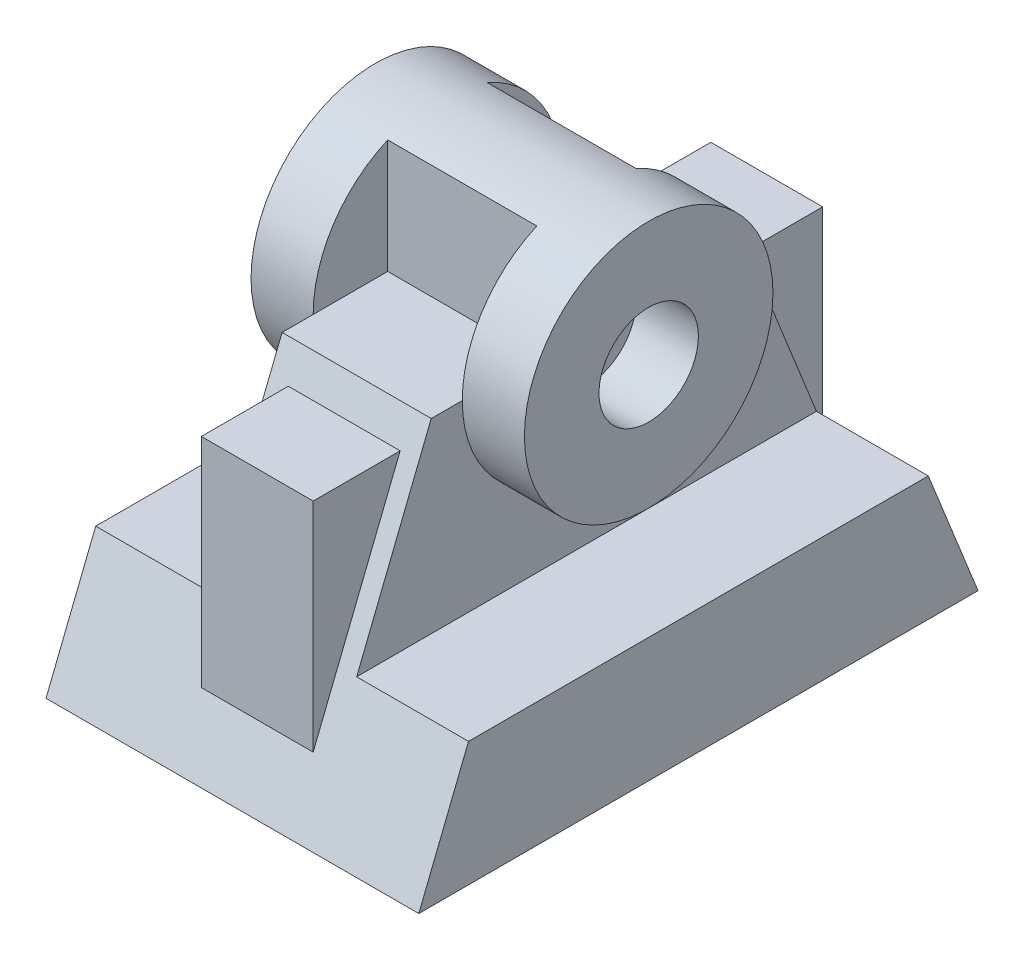
ISO-10303-21;
HEADER;
FILE_DESCRIPTION(('STEP AP214'),'2;1');
FILE_NAME('part.step','',(''),(''),'','','');
FILE_SCHEMA(('AUTOMOTIVE_DESIGN { 1 0 10303 214 1 1 1 1 }'));
ENDSEC;
DATA;
#1=APPLICATION_CONTEXT('core data for automotive mechanical design processes');
#2=APPLICATION_PROTOCOL_DEFINITION('international standard','automotive_design',2000,#1);
#3=PRODUCT_CONTEXT('',#1,'mechanical');
#4=PRODUCT('Part','Part','',(#3));
#5=PRODUCT_RELATED_PRODUCT_CATEGORY('part','',(#4));
#6=PRODUCT_DEFINITION_FORMATION('','',#4);
#7=PRODUCT_DEFINITION_CONTEXT('part definition',#1,'design');
#8=PRODUCT_DEFINITION('design','',#6,#7);
#9=PRODUCT_DEFINITION_SHAPE('','',#8);
#10=(LENGTH_UNIT() NAMED_UNIT(*) SI_UNIT(.MILLI.,.METRE.));
#11=(NAMED_UNIT(*) PLANE_ANGLE_UNIT() SI_UNIT($,.RADIAN.));
#12=(NAMED_UNIT(*) SI_UNIT($,.STERADIAN.) SOLID_ANGLE_UNIT());
#13=UNCERTAINTY_MEASURE_WITH_UNIT(LENGTH_MEASURE(1.E-05),#10,'distance_accuracy_value','');
#14=(GEOMETRIC_REPRESENTATION_CONTEXT(3) GLOBAL_UNCERTAINTY_ASSIGNED_CONTEXT((#13)) GLOBAL_UNIT_ASSIGNED_CONTEXT((#10,
#11,#12)) REPRESENTATION_CONTEXT('',''));
#15=CARTESIAN_POINT('',(0.,0.,0.));
#16=DIRECTION('',(0.,0.,1.));
#17=DIRECTION('',(1.,0.,0.));
#18=AXIS2_PLACEMENT_3D('',#15,#16,#17);
#19=CARTESIAN_POINT('',(22.,50.,0.));
#20=DIRECTION('',(-1.,0.,0.));
#21=DIRECTION('',(0.,0.,1.));
#22=AXIS2_PLACEMENT_3D('',#19,#20,#21);
#23=CYLINDRICAL_SURFACE('',#22,20.);
#24=CARTESIAN_POINT('',(-22.,50.,0.));
#25=DIRECTION('',(1.,0.,0.));
#26=DIRECTION('',(0.,0.,-1.));
#27=AXIS2_PLACEMENT_3D('',#24,#25,#26);
#28=CIRCLE('',#27,20.);
#29=CARTESIAN_POINT('',(-22.,50.,-20.));
#30=VERTEX_POINT('',#29);
#31=EDGE_CURVE('E228',#30,#30,#28,.T.);
#32=ORIENTED_EDGE('',*,*,#31,.T.);
#33=EDGE_LOOP('',(#32));
#34=FACE_BOUND('',#33,.T.);
#35=CARTESIAN_POINT('',(22.,50.,0.));
#36=DIRECTION('',(1.,0.,0.));
#37=DIRECTION('',(0.,0.,-1.));
#38=AXIS2_PLACEMENT_3D('',#35,#36,#37);
#39=CIRCLE('',#38,20.);
#40=CARTESIAN_POINT('',(22.,50.,-20.));
#41=VERTEX_POINT('',#40);
#42=EDGE_CURVE('E226',#41,#41,#39,.T.);
#43=ORIENTED_EDGE('',*,*,#42,.F.);
#44=EDGE_LOOP('',(#43));
#45=FACE_BOUND('',#44,.T.);
#46=CARTESIAN_POINT('',(12.,50.,0.));
#47=DIRECTION('',(-1.,0.,0.));
#48=DIRECTION('',(0.,0.,1.));
#49=AXIS2_PLACEMENT_3D('',#46,#47,#48);
#50=CIRCLE('',#49,20.);
#51=CARTESIAN_POINT('',(12.,68.3303027798234,-8.00000000000001));
#52=VERTEX_POINT('',#51);
#53=CARTESIAN_POINT('',(12.,50.,-20.));
#54=VERTEX_POINT('',#53);
#55=EDGE_CURVE('E199',#52,#54,#50,.T.);
#56=ORIENTED_EDGE('',*,*,#55,.F.);
#57=DIRECTION('',(1.,0.,0.));
#58=VECTOR('',#57,1.);
#59=CARTESIAN_POINT('',(-12.,68.3303027798234,-8.00000000000001));
#60=LINE('',#59,#58);
#61=CARTESIAN_POINT('',(-12.,68.3303027798234,-8.00000000000001));
#62=VERTEX_POINT('',#61);
#63=EDGE_CURVE('E183',#62,#52,#60,.T.);
#64=ORIENTED_EDGE('',*,*,#63,.F.);
#65=CARTESIAN_POINT('',(-12.,50.,0.));
#66=DIRECTION('',(-1.,0.,0.));
#67=DIRECTION('',(0.,0.,1.));
#68=AXIS2_PLACEMENT_3D('',#65,#66,#67);
#69=CIRCLE('',#68,20.);
#70=CARTESIAN_POINT('',(-12.,50.,-20.));
#71=VERTEX_POINT('',#70);
#72=EDGE_CURVE('E53',#62,#71,#69,.T.);
#73=ORIENTED_EDGE('',*,*,#72,.T.);
#74=CARTESIAN_POINT('',(-12.,50.,0.));
#75=DIRECTION('',(1.,0.,0.));
#76=DIRECTION('',(0.,0.,-1.));
#77=AXIS2_PLACEMENT_3D('',#74,#75,#76);
#78=CIRCLE('',#77,20.);
#79=CARTESIAN_POINT('',(-12.,50.,20.));
#80=VERTEX_POINT('',#79);
#81=EDGE_CURVE('E233',#71,#80,#78,.F.);
#82=ORIENTED_EDGE('',*,*,#81,.T.);
#83=CARTESIAN_POINT('',(-12.,50.,0.));
#84=DIRECTION('',(1.,0.,0.));
#85=DIRECTION('',(0.,0.,-1.));
#86=AXIS2_PLACEMENT_3D('',#83,#84,#85);
#87=CIRCLE('',#86,20.);
#88=CARTESIAN_POINT('',(-12.,68.3303027798234,8.00000000000001));
#89=VERTEX_POINT('',#88);
#90=EDGE_CURVE('E210',#89,#80,#87,.T.);
#91=ORIENTED_EDGE('',*,*,#90,.F.);
#92=DIRECTION('',(1.,0.,0.));
#93=VECTOR('',#92,1.);
#94=CARTESIAN_POINT('',(-12.,68.3303027798234,8.00000000000001));
#95=LINE('',#94,#93);
#96=CARTESIAN_POINT('',(12.,68.3303027798234,8.00000000000001));
#97=VERTEX_POINT('',#96);
#98=EDGE_CURVE('E222',#89,#97,#95,.T.);
#99=ORIENTED_EDGE('',*,*,#98,.T.);
#100=CARTESIAN_POINT('',(12.,50.,0.));
#101=DIRECTION('',(1.,0.,0.));
#102=DIRECTION('',(0.,0.,-1.));
#103=AXIS2_PLACEMENT_3D('',#100,#101,#102);
#104=CIRCLE('',#103,20.);
#105=CARTESIAN_POINT('',(12.,50.,20.));
#106=VERTEX_POINT('',#105);
#107=EDGE_CURVE('E195',#97,#106,#104,.T.);
#108=ORIENTED_EDGE('',*,*,#107,.T.);
#109=CARTESIAN_POINT('',(12.,50.,0.));
#110=DIRECTION('',(-1.,0.,0.));
#111=DIRECTION('',(0.,0.,1.));
#112=AXIS2_PLACEMENT_3D('',#109,#110,#111);
#113=CIRCLE('',#112,20.);
#114=EDGE_CURVE('E11',#106,#54,#113,.F.);
#115=ORIENTED_EDGE('',*,*,#114,.T.);
#116=EDGE_LOOP('',(#56,#64,#73,#82,#91,#99,#108,#115));
#117=FACE_BOUND('',#116,.T.);
#118=ADVANCED_FACE('F39',(#34,#45,#117),#23,.T.);
#119=CARTESIAN_POINT('',(30.,50.,25.));
#120=DIRECTION('',(0.,-1.,0.));
#121=DIRECTION('',(0.,0.,-1.));
#122=AXIS2_PLACEMENT_3D('',#119,#120,#121);
#123=PLANE('',#122);
#124=DIRECTION('',(0.,0.,-1.));
#125=VECTOR('',#124,1.);
#126=CARTESIAN_POINT('',(12.,50.,0.));
#127=LINE('',#126,#125);
#128=CARTESIAN_POINT('',(12.,50.,25.));
#129=VERTEX_POINT('',#128);
#130=EDGE_CURVE('E281',#129,#106,#127,.T.);
#131=ORIENTED_EDGE('',*,*,#130,.T.);
#132=DIRECTION('',(0.,0.,-1.));
#133=VECTOR('',#132,1.);
#134=CARTESIAN_POINT('',(12.,50.,8.00000000000001));
#135=LINE('',#134,#133);
#136=CARTESIAN_POINT('',(12.,50.,8.00000000000001));
#137=VERTEX_POINT('',#136);
#138=EDGE_CURVE('E218',#106,#137,#135,.T.);
#139=ORIENTED_EDGE('',*,*,#138,.T.);
#140=DIRECTION('',(1.,0.,0.));
#141=VECTOR('',#140,1.);
#142=CARTESIAN_POINT('',(-12.,50.,8.00000000000001));
#143=LINE('',#142,#141);
#144=CARTESIAN_POINT('',(-12.,50.,8.00000000000001));
#145=VERTEX_POINT('',#144);
#146=EDGE_CURVE('E216',#145,#137,#143,.T.);
#147=ORIENTED_EDGE('',*,*,#146,.F.);
#148=DIRECTION('',(0.,0.,-1.));
#149=VECTOR('',#148,1.);
#150=CARTESIAN_POINT('',(-12.,50.,8.00000000000001));
#151=LINE('',#150,#149);
#152=EDGE_CURVE('E208',#80,#145,#151,.T.);
#153=ORIENTED_EDGE('',*,*,#152,.F.);
#154=DIRECTION('',(0.,0.,1.));
#155=VECTOR('',#154,1.);
#156=CARTESIAN_POINT('',(-12.,50.,0.));
#157=LINE('',#156,#155);
#158=CARTESIAN_POINT('',(-12.,50.,25.));
#159=VERTEX_POINT('',#158);
#160=EDGE_CURVE('E300',#80,#159,#157,.T.);
#161=ORIENTED_EDGE('',*,*,#160,.T.);
#162=DIRECTION('',(-1.,0.,0.));
#163=VECTOR('',#162,1.);
#164=CARTESIAN_POINT('',(30.,50.,25.));
#165=LINE('',#164,#163);
#166=EDGE_CURVE('E335',#129,#159,#165,.T.);
#167=ORIENTED_EDGE('',*,*,#166,.F.);
#168=EDGE_LOOP('',(#131,#139,#147,#153,#161,#167));
#169=FACE_BOUND('',#168,.T.);
#170=ADVANCED_FACE('F374',(#169),#123,.F.);
#171=CARTESIAN_POINT('',(-12.,50.,-25.));
#172=VERTEX_POINT('',#171);
#173=EDGE_CURVE('E182',#172,#71,#157,.T.);
#174=ORIENTED_EDGE('',*,*,#173,.T.);
#175=DIRECTION('',(0.,0.,1.));
#176=VECTOR('',#175,1.);
#177=CARTESIAN_POINT('',(-12.,50.,-8.00000000000001));
#178=LINE('',#177,#176);
#179=CARTESIAN_POINT('',(-12.,50.,-8.00000000000001));
#180=VERTEX_POINT('',#179);
#181=EDGE_CURVE('E180',#71,#180,#178,.T.);
#182=ORIENTED_EDGE('',*,*,#181,.T.);
#183=DIRECTION('',(1.,0.,0.));
#184=VECTOR('',#183,1.);
#185=CARTESIAN_POINT('',(-12.,50.,-8.00000000000001));
#186=LINE('',#185,#184);
#187=CARTESIAN_POINT('',(12.,50.,-8.00000000000001));
#188=VERTEX_POINT('',#187);
#189=EDGE_CURVE('E179',#180,#188,#186,.T.);
#190=ORIENTED_EDGE('',*,*,#189,.T.);
#191=DIRECTION('',(0.,0.,1.));
#192=VECTOR('',#191,1.);
#193=CARTESIAN_POINT('',(12.,50.,-8.00000000000001));
#194=LINE('',#193,#192);
#195=EDGE_CURVE('E196',#54,#188,#194,.T.);
#196=ORIENTED_EDGE('',*,*,#195,.F.);
#197=CARTESIAN_POINT('',(12.,50.,-25.));
#198=VERTEX_POINT('',#197);
#199=EDGE_CURVE('E278',#54,#198,#127,.T.);
#200=ORIENTED_EDGE('',*,*,#199,.T.);
#201=DIRECTION('',(-1.,0.,0.));
#202=VECTOR('',#201,1.);
#203=CARTESIAN_POINT('',(30.,50.,-25.));
#204=LINE('',#203,#202);
#205=EDGE_CURVE('E334',#198,#172,#204,.T.);
#206=ORIENTED_EDGE('',*,*,#205,.T.);
#207=EDGE_LOOP('',(#174,#182,#190,#196,#200,#206));
#208=FACE_BOUND('',#207,.T.);
#209=ADVANCED_FACE('F177',(#208),#123,.F.);
#210=CARTESIAN_POINT('',(30.,0.,0.));
#211=DIRECTION('',(1.,0.,0.));
#212=DIRECTION('',(0.,0.,-1.));
#213=AXIS2_PLACEMENT_3D('',#210,#211,#212);
#214=PLANE('',#213);
#215=DIRECTION('',(0.,0.928476690885259,0.371390676354104));
#216=VECTOR('',#215,1.);
#217=CARTESIAN_POINT('',(30.,0.,-45.));
#218=LINE('',#217,#216);
#219=CARTESIAN_POINT('',(30.,0.,-45.));
#220=VERTEX_POINT('',#219);
#221=CARTESIAN_POINT('',(30.,20.,-37.));
#222=VERTEX_POINT('',#221);
#223=EDGE_CURVE('E312',#220,#222,#218,.T.);
#224=ORIENTED_EDGE('',*,*,#223,.T.);
#225=DIRECTION('',(0.,0.,1.));
#226=VECTOR('',#225,1.);
#227=CARTESIAN_POINT('',(30.,20.,0.));
#228=LINE('',#227,#226);
#229=CARTESIAN_POINT('',(30.,20.,37.));
#230=VERTEX_POINT('',#229);
#231=EDGE_CURVE('E271',#222,#230,#228,.T.);
#232=ORIENTED_EDGE('',*,*,#231,.T.);
#233=DIRECTION('',(0.,-0.928476690885259,0.371390676354104));
#234=VECTOR('',#233,1.);
#235=CARTESIAN_POINT('',(30.,0.,45.));
#236=LINE('',#235,#234);
#237=CARTESIAN_POINT('',(30.,0.,45.));
#238=VERTEX_POINT('',#237);
#239=EDGE_CURVE('E317',#230,#238,#236,.T.);
#240=ORIENTED_EDGE('',*,*,#239,.T.);
#241=DIRECTION('',(0.,0.,-1.));
#242=VECTOR('',#241,1.);
#243=CARTESIAN_POINT('',(30.,0.,45.));
#244=LINE('',#243,#242);
#245=EDGE_CURVE('E316',#238,#220,#244,.T.);
#246=ORIENTED_EDGE('',*,*,#245,.T.);
#247=EDGE_LOOP('',(#224,#232,#240,#246));
#248=FACE_BOUND('',#247,.T.);
#249=ADVANCED_FACE('F428',(#248),#214,.T.);
#250=CARTESIAN_POINT('',(30.,0.,-45.));
#251=DIRECTION('',(0.,-0.371390676354104,0.928476690885259));
#252=DIRECTION('',(0.,-0.928476690885259,-0.371390676354104));
#253=AXIS2_PLACEMENT_3D('',#250,#251,#252);
#254=PLANE('',#253);
#255=DIRECTION('',(-1.,0.,0.));
#256=VECTOR('',#255,1.);
#257=CARTESIAN_POINT('',(9.,9.99999999999999,-41.));
#258=LINE('',#257,#256);
#259=CARTESIAN_POINT('',(9.,10.,-41.));
#260=VERTEX_POINT('',#259);
#261=CARTESIAN_POINT('',(-9.,9.99999999999999,-41.));
#262=VERTEX_POINT('',#261);
#263=EDGE_CURVE('E258',#260,#262,#258,.T.);
#264=ORIENTED_EDGE('',*,*,#263,.F.);
#265=DIRECTION('',(0.,0.928476690885259,0.371390676354104));
#266=VECTOR('',#265,1.);
#267=CARTESIAN_POINT('',(9.,0.,-45.));
#268=LINE('',#267,#266);
#269=CARTESIAN_POINT('',(9.,45.,-27.));
#270=VERTEX_POINT('',#269);
#271=EDGE_CURVE('E267',#260,#270,#268,.T.);
#272=ORIENTED_EDGE('',*,*,#271,.T.);
#273=DIRECTION('',(1.,0.,0.));
#274=VECTOR('',#273,1.);
#275=CARTESIAN_POINT('',(30.,45.,-27.));
#276=LINE('',#275,#274);
#277=CARTESIAN_POINT('',(-9.,45.,-27.));
#278=VERTEX_POINT('',#277);
#279=EDGE_CURVE('E269',#278,#270,#276,.T.);
#280=ORIENTED_EDGE('',*,*,#279,.F.);
#281=DIRECTION('',(0.,0.928476690885259,0.371390676354104));
#282=VECTOR('',#281,1.);
#283=CARTESIAN_POINT('',(-9.,0.,-45.));
#284=LINE('',#283,#282);
#285=EDGE_CURVE('E264',#262,#278,#284,.T.);
#286=ORIENTED_EDGE('',*,*,#285,.F.);
#287=EDGE_LOOP('',(#264,#272,#280,#286));
#288=FACE_BOUND('',#287,.T.);
#289=DIRECTION('',(0.,-0.928476690885259,-0.371390676354104));
#290=VECTOR('',#289,1.);
#291=CARTESIAN_POINT('',(12.,15.5172413793103,-38.7931034482759));
#292=LINE('',#291,#290);
#293=CARTESIAN_POINT('',(12.,20.,-37.));
#294=VERTEX_POINT('',#293);
#295=EDGE_CURVE('E283',#198,#294,#292,.T.);
#296=ORIENTED_EDGE('',*,*,#295,.T.);
#297=DIRECTION('',(1.,0.,0.));
#298=VECTOR('',#297,1.);
#299=CARTESIAN_POINT('',(12.,20.,-37.));
#300=LINE('',#299,#298);
#301=EDGE_CURVE('E290',#294,#222,#300,.T.);
#302=ORIENTED_EDGE('',*,*,#301,.T.);
#303=ORIENTED_EDGE('',*,*,#223,.F.);
#304=DIRECTION('',(-1.,0.,0.));
#305=VECTOR('',#304,1.);
#306=CARTESIAN_POINT('',(30.,0.,-45.));
#307=LINE('',#306,#305);
#308=CARTESIAN_POINT('',(-30.,0.,-45.));
#309=VERTEX_POINT('',#308);
#310=EDGE_CURVE('E322',#220,#309,#307,.T.);
#311=ORIENTED_EDGE('',*,*,#310,.T.);
#312=DIRECTION('',(0.,0.928476690885259,0.371390676354104));
#313=VECTOR('',#312,1.);
#314=CARTESIAN_POINT('',(-30.,0.,-45.));
#315=LINE('',#314,#313);
#316=CARTESIAN_POINT('',(-30.,20.,-37.));
#317=VERTEX_POINT('',#316);
#318=EDGE_CURVE('E315',#309,#317,#315,.T.);
#319=ORIENTED_EDGE('',*,*,#318,.T.);
#320=DIRECTION('',(-1.,0.,0.));
#321=VECTOR('',#320,1.);
#322=CARTESIAN_POINT('',(-12.,20.,-37.));
#323=LINE('',#322,#321);
#324=CARTESIAN_POINT('',(-12.,20.,-37.));
#325=VERTEX_POINT('',#324);
#326=EDGE_CURVE('E304',#325,#317,#323,.T.);
#327=ORIENTED_EDGE('',*,*,#326,.F.);
#328=DIRECTION('',(0.,0.928476690885259,0.371390676354104));
#329=VECTOR('',#328,1.);
#330=CARTESIAN_POINT('',(-12.,15.5172413793103,-38.7931034482759));
#331=LINE('',#330,#329);
#332=EDGE_CURVE('E305',#325,#172,#331,.T.);
#333=ORIENTED_EDGE('',*,*,#332,.T.);
#334=ORIENTED_EDGE('',*,*,#205,.F.);
#335=EDGE_LOOP('',(#296,#302,#303,#311,#319,#327,#333,#334));
#336=FACE_BOUND('',#335,.T.);
#337=ADVANCED_FACE('F41',(#288,#336),#254,.F.);
#338=CARTESIAN_POINT('',(30.,0.,45.));
#339=DIRECTION('',(0.,-0.371390676354104,-0.928476690885259));
#340=DIRECTION('',(0.,0.928476690885259,-0.371390676354104));
#341=AXIS2_PLACEMENT_3D('',#338,#339,#340);
#342=PLANE('',#341);
#343=DIRECTION('',(-1.,0.,0.));
#344=VECTOR('',#343,1.);
#345=CARTESIAN_POINT('',(30.,45.,27.));
#346=LINE('',#345,#344);
#347=CARTESIAN_POINT('',(9.,45.,27.));
#348=VERTEX_POINT('',#347);
#349=CARTESIAN_POINT('',(-9.,45.,27.));
#350=VERTEX_POINT('',#349);
#351=EDGE_CURVE('E338',#348,#350,#346,.T.);
#352=ORIENTED_EDGE('',*,*,#351,.F.);
#353=DIRECTION('',(0.,-0.928476690885259,0.371390676354104));
#354=VECTOR('',#353,1.);
#355=CARTESIAN_POINT('',(9.,0.,45.));
#356=LINE('',#355,#354);
#357=CARTESIAN_POINT('',(9.,9.99999999999999,41.));
#358=VERTEX_POINT('',#357);
#359=EDGE_CURVE('E50',#348,#358,#356,.T.);
#360=ORIENTED_EDGE('',*,*,#359,.T.);
#361=DIRECTION('',(-1.,0.,0.));
#362=VECTOR('',#361,1.);
#363=CARTESIAN_POINT('',(9.,9.99999999999999,41.));
#364=LINE('',#363,#362);
#365=CARTESIAN_POINT('',(-9.,9.99999999999999,41.));
#366=VERTEX_POINT('',#365);
#367=EDGE_CURVE('E262',#358,#366,#364,.T.);
#368=ORIENTED_EDGE('',*,*,#367,.T.);
#369=DIRECTION('',(0.,-0.928476690885259,0.371390676354104));
#370=VECTOR('',#369,1.);
#371=CARTESIAN_POINT('',(-9.,0.,45.));
#372=LINE('',#371,#370);
#373=EDGE_CURVE('E340',#350,#366,#372,.T.);
#374=ORIENTED_EDGE('',*,*,#373,.F.);
#375=EDGE_LOOP('',(#352,#360,#368,#374));
#376=FACE_BOUND('',#375,.T.);
#377=DIRECTION('',(1.,0.,0.));
#378=VECTOR('',#377,1.);
#379=CARTESIAN_POINT('',(12.,20.,37.));
#380=LINE('',#379,#378);
#381=CARTESIAN_POINT('',(12.,20.,37.));
#382=VERTEX_POINT('',#381);
#383=EDGE_CURVE('E292',#382,#230,#380,.T.);
#384=ORIENTED_EDGE('',*,*,#383,.F.);
#385=DIRECTION('',(0.,0.928476690885259,-0.371390676354104));
#386=VECTOR('',#385,1.);
#387=CARTESIAN_POINT('',(12.,15.5172413793104,38.7931034482759));
#388=LINE('',#387,#386);
#389=EDGE_CURVE('E280',#382,#129,#388,.T.);
#390=ORIENTED_EDGE('',*,*,#389,.T.);
#391=ORIENTED_EDGE('',*,*,#166,.T.);
#392=DIRECTION('',(0.,-0.928476690885259,0.371390676354104));
#393=VECTOR('',#392,1.);
#394=CARTESIAN_POINT('',(-12.,15.5172413793104,38.7931034482759));
#395=LINE('',#394,#393);
#396=CARTESIAN_POINT('',(-12.,20.,37.));
#397=VERTEX_POINT('',#396);
#398=EDGE_CURVE('E298',#159,#397,#395,.T.);
#399=ORIENTED_EDGE('',*,*,#398,.T.);
#400=DIRECTION('',(-1.,0.,0.));
#401=VECTOR('',#400,1.);
#402=CARTESIAN_POINT('',(-12.,20.,37.));
#403=LINE('',#402,#401);
#404=CARTESIAN_POINT('',(-30.,20.,37.));
#405=VERTEX_POINT('',#404);
#406=EDGE_CURVE('E307',#397,#405,#403,.T.);
#407=ORIENTED_EDGE('',*,*,#406,.T.);
#408=DIRECTION('',(0.,-0.928476690885259,0.371390676354104));
#409=VECTOR('',#408,1.);
#410=CARTESIAN_POINT('',(-30.,0.,45.));
#411=LINE('',#410,#409);
#412=CARTESIAN_POINT('',(-30.,0.,45.));
#413=VERTEX_POINT('',#412);
#414=EDGE_CURVE('E321',#405,#413,#411,.T.);
#415=ORIENTED_EDGE('',*,*,#414,.T.);
#416=DIRECTION('',(-1.,0.,0.));
#417=VECTOR('',#416,1.);
#418=CARTESIAN_POINT('',(30.,0.,45.));
#419=LINE('',#418,#417);
#420=EDGE_CURVE('E328',#238,#413,#419,.T.);
#421=ORIENTED_EDGE('',*,*,#420,.F.);
#422=ORIENTED_EDGE('',*,*,#239,.F.);
#423=EDGE_LOOP('',(#384,#390,#391,#399,#407,#415,#421,#422));
#424=FACE_BOUND('',#423,.T.);
#425=ADVANCED_FACE('F341',(#376,#424),#342,.F.);
#426=CARTESIAN_POINT('',(30.,0.,45.));
#427=DIRECTION('',(0.,1.,0.));
#428=DIRECTION('',(0.,0.,1.));
#429=AXIS2_PLACEMENT_3D('',#426,#427,#428);
#430=PLANE('',#429);
#431=DIRECTION('',(0.,0.,-1.));
#432=VECTOR('',#431,1.);
#433=CARTESIAN_POINT('',(-30.,0.,45.));
#434=LINE('',#433,#432);
#435=EDGE_CURVE('E320',#413,#309,#434,.T.);
#436=ORIENTED_EDGE('',*,*,#435,.T.);
#437=ORIENTED_EDGE('',*,*,#310,.F.);
#438=ORIENTED_EDGE('',*,*,#245,.F.);
#439=ORIENTED_EDGE('',*,*,#420,.T.);
#440=EDGE_LOOP('',(#436,#437,#438,#439));
#441=FACE_BOUND('',#440,.T.);
#442=ADVANCED_FACE('F435',(#441),#430,.F.);
#443=CARTESIAN_POINT('',(-30.,0.,0.));
#444=DIRECTION('',(1.,0.,0.));
#445=DIRECTION('',(0.,0.,-1.));
#446=AXIS2_PLACEMENT_3D('',#443,#444,#445);
#447=PLANE('',#446);
#448=ORIENTED_EDGE('',*,*,#414,.F.);
#449=DIRECTION('',(0.,0.,-1.));
#450=VECTOR('',#449,1.);
#451=CARTESIAN_POINT('',(-30.,20.,0.));
#452=LINE('',#451,#450);
#453=EDGE_CURVE('E295',#405,#317,#452,.T.);
#454=ORIENTED_EDGE('',*,*,#453,.T.);
#455=ORIENTED_EDGE('',*,*,#318,.F.);
#456=ORIENTED_EDGE('',*,*,#435,.F.);
#457=EDGE_LOOP('',(#448,#454,#455,#456));
#458=FACE_BOUND('',#457,.T.);
#459=ADVANCED_FACE('F425',(#458),#447,.F.);
#460=CARTESIAN_POINT('',(-12.,20.,0.));
#461=DIRECTION('',(0.,1.,0.));
#462=DIRECTION('',(0.,0.,1.));
#463=AXIS2_PLACEMENT_3D('',#460,#461,#462);
#464=PLANE('',#463);
#465=ORIENTED_EDGE('',*,*,#453,.F.);
#466=ORIENTED_EDGE('',*,*,#406,.F.);
#467=DIRECTION('',(0.,0.,-1.));
#468=VECTOR('',#467,1.);
#469=CARTESIAN_POINT('',(-12.,20.,0.));
#470=LINE('',#469,#468);
#471=EDGE_CURVE('E297',#397,#325,#470,.T.);
#472=ORIENTED_EDGE('',*,*,#471,.T.);
#473=ORIENTED_EDGE('',*,*,#326,.T.);
#474=EDGE_LOOP('',(#465,#466,#472,#473));
#475=FACE_BOUND('',#474,.T.);
#476=ADVANCED_FACE('F419',(#475),#464,.T.);
#477=CARTESIAN_POINT('',(-12.,0.,0.));
#478=DIRECTION('',(1.,0.,0.));
#479=DIRECTION('',(0.,0.,-1.));
#480=AXIS2_PLACEMENT_3D('',#477,#478,#479);
#481=PLANE('',#480);
#482=ORIENTED_EDGE('',*,*,#81,.F.);
#483=ORIENTED_EDGE('',*,*,#173,.F.);
#484=ORIENTED_EDGE('',*,*,#332,.F.);
#485=ORIENTED_EDGE('',*,*,#471,.F.);
#486=ORIENTED_EDGE('',*,*,#398,.F.);
#487=ORIENTED_EDGE('',*,*,#160,.F.);
#488=EDGE_LOOP('',(#482,#483,#484,#485,#486,#487));
#489=FACE_BOUND('',#488,.T.);
#490=ADVANCED_FACE('F413',(#489),#481,.F.);
#491=CARTESIAN_POINT('',(12.,20.,0.));
#492=DIRECTION('',(0.,1.,0.));
#493=DIRECTION('',(0.,0.,1.));
#494=AXIS2_PLACEMENT_3D('',#491,#492,#493);
#495=PLANE('',#494);
#496=ORIENTED_EDGE('',*,*,#231,.F.);
#497=ORIENTED_EDGE('',*,*,#301,.F.);
#498=DIRECTION('',(0.,0.,1.));
#499=VECTOR('',#498,1.);
#500=CARTESIAN_POINT('',(12.,20.,0.));
#501=LINE('',#500,#499);
#502=EDGE_CURVE('E274',#294,#382,#501,.T.);
#503=ORIENTED_EDGE('',*,*,#502,.T.);
#504=ORIENTED_EDGE('',*,*,#383,.T.);
#505=EDGE_LOOP('',(#496,#497,#503,#504));
#506=FACE_BOUND('',#505,.T.);
#507=ADVANCED_FACE('F407',(#506),#495,.T.);
#508=CARTESIAN_POINT('',(12.,0.,0.));
#509=DIRECTION('',(-1.,0.,0.));
#510=DIRECTION('',(0.,0.,1.));
#511=AXIS2_PLACEMENT_3D('',#508,#509,#510);
#512=PLANE('',#511);
#513=ORIENTED_EDGE('',*,*,#114,.F.);
#514=ORIENTED_EDGE('',*,*,#130,.F.);
#515=ORIENTED_EDGE('',*,*,#389,.F.);
#516=ORIENTED_EDGE('',*,*,#502,.F.);
#517=ORIENTED_EDGE('',*,*,#295,.F.);
#518=ORIENTED_EDGE('',*,*,#199,.F.);
#519=EDGE_LOOP('',(#513,#514,#515,#516,#517,#518));
#520=FACE_BOUND('',#519,.T.);
#521=ADVANCED_FACE('F402',(#520),#512,.F.);
#522=CARTESIAN_POINT('',(-9.,0.,0.));
#523=DIRECTION('',(1.,0.,0.));
#524=DIRECTION('',(0.,0.,-1.));
#525=AXIS2_PLACEMENT_3D('',#522,#523,#524);
#526=PLANE('',#525);
#527=DIRECTION('',(0.,0.,1.));
#528=VECTOR('',#527,1.);
#529=CARTESIAN_POINT('',(-9.,45.,41.));
#530=LINE('',#529,#528);
#531=CARTESIAN_POINT('',(-9.,45.,41.));
#532=VERTEX_POINT('',#531);
#533=EDGE_CURVE('E255',#350,#532,#530,.T.);
#534=ORIENTED_EDGE('',*,*,#533,.F.);
#535=ORIENTED_EDGE('',*,*,#373,.T.);
#536=DIRECTION('',(0.,-1.,0.));
#537=VECTOR('',#536,1.);
#538=CARTESIAN_POINT('',(-9.,45.,41.));
#539=LINE('',#538,#537);
#540=EDGE_CURVE('E236',#532,#366,#539,.T.);
#541=ORIENTED_EDGE('',*,*,#540,.F.);
#542=EDGE_LOOP('',(#534,#535,#541));
#543=FACE_BOUND('',#542,.T.);
#544=ADVANCED_FACE('F357',(#543),#526,.F.);
#545=CARTESIAN_POINT('',(9.,0.,0.));
#546=DIRECTION('',(1.,0.,0.));
#547=DIRECTION('',(0.,0.,-1.));
#548=AXIS2_PLACEMENT_3D('',#545,#546,#547);
#549=PLANE('',#548);
#550=ORIENTED_EDGE('',*,*,#359,.F.);
#551=DIRECTION('',(0.,0.,1.));
#552=VECTOR('',#551,1.);
#553=CARTESIAN_POINT('',(9.,45.,41.));
#554=LINE('',#553,#552);
#555=CARTESIAN_POINT('',(9.,45.,41.));
#556=VERTEX_POINT('',#555);
#557=EDGE_CURVE('E243',#348,#556,#554,.T.);
#558=ORIENTED_EDGE('',*,*,#557,.T.);
#559=DIRECTION('',(0.,-1.,0.));
#560=VECTOR('',#559,1.);
#561=CARTESIAN_POINT('',(9.,45.,41.));
#562=LINE('',#561,#560);
#563=EDGE_CURVE('E240',#556,#358,#562,.T.);
#564=ORIENTED_EDGE('',*,*,#563,.T.);
#565=EDGE_LOOP('',(#550,#558,#564));
#566=FACE_BOUND('',#565,.T.);
#567=ADVANCED_FACE('F349',(#566),#549,.T.);
#568=CARTESIAN_POINT('',(9.,45.,41.));
#569=DIRECTION('',(0.,-1.,0.));
#570=DIRECTION('',(0.,0.,-1.));
#571=AXIS2_PLACEMENT_3D('',#568,#569,#570);
#572=PLANE('',#571);
#573=ORIENTED_EDGE('',*,*,#557,.F.);
#574=ORIENTED_EDGE('',*,*,#351,.T.);
#575=ORIENTED_EDGE('',*,*,#533,.T.);
#576=DIRECTION('',(-1.,0.,0.));
#577=VECTOR('',#576,1.);
#578=CARTESIAN_POINT('',(9.,45.,41.));
#579=LINE('',#578,#577);
#580=EDGE_CURVE('E250',#556,#532,#579,.T.);
#581=ORIENTED_EDGE('',*,*,#580,.F.);
#582=EDGE_LOOP('',(#573,#574,#575,#581));
#583=FACE_BOUND('',#582,.T.);
#584=ADVANCED_FACE('F360',(#583),#572,.F.);
#585=CARTESIAN_POINT('',(9.,45.,41.));
#586=DIRECTION('',(0.,0.,-1.));
#587=DIRECTION('',(0.,1.,0.));
#588=AXIS2_PLACEMENT_3D('',#585,#586,#587);
#589=PLANE('',#588);
#590=ORIENTED_EDGE('',*,*,#540,.T.);
#591=ORIENTED_EDGE('',*,*,#367,.F.);
#592=ORIENTED_EDGE('',*,*,#563,.F.);
#593=ORIENTED_EDGE('',*,*,#580,.T.);
#594=EDGE_LOOP('',(#590,#591,#592,#593));
#595=FACE_BOUND('',#594,.T.);
#596=ADVANCED_FACE('F352',(#595),#589,.F.);
#597=CARTESIAN_POINT('',(-9.,45.,-41.));
#598=VERTEX_POINT('',#597);
#599=EDGE_CURVE('E241',#598,#278,#530,.T.);
#600=ORIENTED_EDGE('',*,*,#599,.T.);
#601=ORIENTED_EDGE('',*,*,#279,.T.);
#602=CARTESIAN_POINT('',(9.,45.,-41.));
#603=VERTEX_POINT('',#602);
#604=EDGE_CURVE('E242',#603,#270,#554,.T.);
#605=ORIENTED_EDGE('',*,*,#604,.F.);
#606=DIRECTION('',(-1.,0.,0.));
#607=VECTOR('',#606,1.);
#608=CARTESIAN_POINT('',(9.,45.,-41.));
#609=LINE('',#608,#607);
#610=EDGE_CURVE('E260',#603,#598,#609,.T.);
#611=ORIENTED_EDGE('',*,*,#610,.T.);
#612=EDGE_LOOP('',(#600,#601,#605,#611));
#613=FACE_BOUND('',#612,.T.);
#614=ADVANCED_FACE('F365',(#613),#572,.F.);
#615=ORIENTED_EDGE('',*,*,#271,.F.);
#616=DIRECTION('',(0.,1.,0.));
#617=VECTOR('',#616,1.);
#618=CARTESIAN_POINT('',(9.,45.,-41.));
#619=LINE('',#618,#617);
#620=EDGE_CURVE('E239',#260,#603,#619,.T.);
#621=ORIENTED_EDGE('',*,*,#620,.T.);
#622=ORIENTED_EDGE('',*,*,#604,.T.);
#623=EDGE_LOOP('',(#615,#621,#622));
#624=FACE_BOUND('',#623,.T.);
#625=ADVANCED_FACE('F367',(#624),#549,.T.);
#626=DIRECTION('',(0.,1.,0.));
#627=VECTOR('',#626,1.);
#628=CARTESIAN_POINT('',(-9.,45.,-41.));
#629=LINE('',#628,#627);
#630=EDGE_CURVE('E249',#262,#598,#629,.T.);
#631=ORIENTED_EDGE('',*,*,#630,.F.);
#632=ORIENTED_EDGE('',*,*,#285,.T.);
#633=ORIENTED_EDGE('',*,*,#599,.F.);
#634=EDGE_LOOP('',(#631,#632,#633));
#635=FACE_BOUND('',#634,.T.);
#636=ADVANCED_FACE('F386',(#635),#526,.F.);
#637=CARTESIAN_POINT('',(9.,45.,-41.));
#638=DIRECTION('',(0.,0.,1.));
#639=DIRECTION('',(0.,-1.,0.));
#640=AXIS2_PLACEMENT_3D('',#637,#638,#639);
#641=PLANE('',#640);
#642=ORIENTED_EDGE('',*,*,#630,.T.);
#643=ORIENTED_EDGE('',*,*,#610,.F.);
#644=ORIENTED_EDGE('',*,*,#620,.F.);
#645=ORIENTED_EDGE('',*,*,#263,.T.);
#646=EDGE_LOOP('',(#642,#643,#644,#645));
#647=FACE_BOUND('',#646,.T.);
#648=ADVANCED_FACE('F395',(#647),#641,.F.);
#649=CARTESIAN_POINT('',(22.,50.,0.));
#650=DIRECTION('',(1.,0.,0.));
#651=DIRECTION('',(0.,0.,-1.));
#652=AXIS2_PLACEMENT_3D('',#649,#650,#651);
#653=PLANE('',#652);
#654=CARTESIAN_POINT('',(22.,50.,0.));
#655=DIRECTION('',(1.,0.,0.));
#656=DIRECTION('',(0.,0.,-1.));
#657=AXIS2_PLACEMENT_3D('',#654,#655,#656);
#658=CIRCLE('',#657,8.);
#659=CARTESIAN_POINT('',(22.,50.,-8.));
#660=VERTEX_POINT('',#659);
#661=EDGE_CURVE('E501',#660,#660,#658,.T.);
#662=ORIENTED_EDGE('',*,*,#661,.F.);
#663=EDGE_LOOP('',(#662));
#664=FACE_BOUND('',#663,.T.);
#665=ORIENTED_EDGE('',*,*,#42,.T.);
#666=EDGE_LOOP('',(#665));
#667=FACE_BOUND('',#666,.T.);
#668=ADVANCED_FACE('F400',(#664,#667),#653,.T.);
#669=CARTESIAN_POINT('',(-22.,50.,0.));
#670=DIRECTION('',(1.,0.,0.));
#671=DIRECTION('',(0.,0.,-1.));
#672=AXIS2_PLACEMENT_3D('',#669,#670,#671);
#673=PLANE('',#672);
#674=CARTESIAN_POINT('',(-22.,50.,0.));
#675=DIRECTION('',(1.,0.,0.));
#676=DIRECTION('',(0.,0.,-1.));
#677=AXIS2_PLACEMENT_3D('',#674,#675,#676);
#678=CIRCLE('',#677,8.);
#679=CARTESIAN_POINT('',(-22.,50.,-8.));
#680=VERTEX_POINT('',#679);
#681=EDGE_CURVE('E507',#680,#680,#678,.T.);
#682=ORIENTED_EDGE('',*,*,#681,.T.);
#683=EDGE_LOOP('',(#682));
#684=FACE_BOUND('',#683,.T.);
#685=ORIENTED_EDGE('',*,*,#31,.F.);
#686=EDGE_LOOP('',(#685));
#687=FACE_BOUND('',#686,.T.);
#688=ADVANCED_FACE('F387',(#684,#687),#673,.F.);
#689=CARTESIAN_POINT('',(-12.,68.3303027798234,8.00000000000001));
#690=DIRECTION('',(0.,0.,-1.));
#691=DIRECTION('',(0.,1.,0.));
#692=AXIS2_PLACEMENT_3D('',#689,#690,#691);
#693=PLANE('',#692);
#694=DIRECTION('',(0.,1.,0.));
#695=VECTOR('',#694,1.);
#696=CARTESIAN_POINT('',(12.,68.3303027798234,8.00000000000001));
#697=LINE('',#696,#695);
#698=EDGE_CURVE('E65',#137,#97,#697,.T.);
#699=ORIENTED_EDGE('',*,*,#698,.T.);
#700=ORIENTED_EDGE('',*,*,#98,.F.);
#701=DIRECTION('',(0.,1.,0.));
#702=VECTOR('',#701,1.);
#703=CARTESIAN_POINT('',(-12.,68.3303027798234,8.00000000000001));
#704=LINE('',#703,#702);
#705=EDGE_CURVE('E214',#145,#89,#704,.T.);
#706=ORIENTED_EDGE('',*,*,#705,.F.);
#707=ORIENTED_EDGE('',*,*,#146,.T.);
#708=EDGE_LOOP('',(#699,#700,#706,#707));
#709=FACE_BOUND('',#708,.T.);
#710=ADVANCED_FACE('F486',(#709),#693,.F.);
#711=CARTESIAN_POINT('',(-12.,50.,0.));
#712=DIRECTION('',(1.,0.,0.));
#713=DIRECTION('',(0.,0.,-1.));
#714=AXIS2_PLACEMENT_3D('',#711,#712,#713);
#715=PLANE('',#714);
#716=ORIENTED_EDGE('',*,*,#90,.T.);
#717=ORIENTED_EDGE('',*,*,#152,.T.);
#718=ORIENTED_EDGE('',*,*,#705,.T.);
#719=EDGE_LOOP('',(#716,#717,#718));
#720=FACE_BOUND('',#719,.T.);
#721=ADVANCED_FACE('F484',(#720),#715,.T.);
#722=CARTESIAN_POINT('',(12.,50.,0.));
#723=DIRECTION('',(1.,0.,0.));
#724=DIRECTION('',(0.,0.,-1.));
#725=AXIS2_PLACEMENT_3D('',#722,#723,#724);
#726=PLANE('',#725);
#727=ORIENTED_EDGE('',*,*,#107,.F.);
#728=ORIENTED_EDGE('',*,*,#698,.F.);
#729=ORIENTED_EDGE('',*,*,#138,.F.);
#730=EDGE_LOOP('',(#727,#728,#729));
#731=FACE_BOUND('',#730,.T.);
#732=ADVANCED_FACE('F483',(#731),#726,.F.);
#733=CARTESIAN_POINT('',(-12.,68.3303027798234,-8.00000000000001));
#734=DIRECTION('',(0.,0.,-1.));
#735=DIRECTION('',(0.,1.,0.));
#736=AXIS2_PLACEMENT_3D('',#733,#734,#735);
#737=PLANE('',#736);
#738=DIRECTION('',(0.,1.,0.));
#739=VECTOR('',#738,1.);
#740=CARTESIAN_POINT('',(12.,68.3303027798234,-8.00000000000001));
#741=LINE('',#740,#739);
#742=EDGE_CURVE('E192',#188,#52,#741,.T.);
#743=ORIENTED_EDGE('',*,*,#742,.F.);
#744=ORIENTED_EDGE('',*,*,#189,.F.);
#745=DIRECTION('',(0.,1.,0.));
#746=VECTOR('',#745,1.);
#747=CARTESIAN_POINT('',(-12.,68.3303027798234,-8.00000000000001));
#748=LINE('',#747,#746);
#749=EDGE_CURVE('E184',#180,#62,#748,.T.);
#750=ORIENTED_EDGE('',*,*,#749,.T.);
#751=ORIENTED_EDGE('',*,*,#63,.T.);
#752=EDGE_LOOP('',(#743,#744,#750,#751));
#753=FACE_BOUND('',#752,.T.);
#754=ADVANCED_FACE('F189',(#753),#737,.T.);
#755=CARTESIAN_POINT('',(-12.,50.,0.));
#756=DIRECTION('',(1.,0.,0.));
#757=DIRECTION('',(0.,0.,1.));
#758=AXIS2_PLACEMENT_3D('',#755,#756,#757);
#759=PLANE('',#758);
#760=ORIENTED_EDGE('',*,*,#72,.F.);
#761=ORIENTED_EDGE('',*,*,#749,.F.);
#762=ORIENTED_EDGE('',*,*,#181,.F.);
#763=EDGE_LOOP('',(#760,#761,#762));
#764=FACE_BOUND('',#763,.T.);
#765=ADVANCED_FACE('F191',(#764),#759,.T.);
#766=CARTESIAN_POINT('',(12.,50.,0.));
#767=DIRECTION('',(1.,0.,0.));
#768=DIRECTION('',(0.,0.,1.));
#769=AXIS2_PLACEMENT_3D('',#766,#767,#768);
#770=PLANE('',#769);
#771=ORIENTED_EDGE('',*,*,#55,.T.);
#772=ORIENTED_EDGE('',*,*,#195,.T.);
#773=ORIENTED_EDGE('',*,*,#742,.T.);
#774=EDGE_LOOP('',(#771,#772,#773));
#775=FACE_BOUND('',#774,.T.);
#776=ADVANCED_FACE('F469',(#775),#770,.F.);
#777=CARTESIAN_POINT('',(12.01,50.,0.));
#778=DIRECTION('',(1.,0.,0.));
#779=DIRECTION('',(0.,0.,-1.));
#780=AXIS2_PLACEMENT_3D('',#777,#778,#779);
#781=CYLINDRICAL_SURFACE('',#780,8.);
#782=CARTESIAN_POINT('',(12.01,50.,0.));
#783=DIRECTION('',(1.,0.,0.));
#784=DIRECTION('',(0.,0.,-1.));
#785=AXIS2_PLACEMENT_3D('',#782,#783,#784);
#786=CIRCLE('',#785,8.);
#787=CARTESIAN_POINT('',(12.01,50.,-8.));
#788=VERTEX_POINT('',#787);
#789=EDGE_CURVE('E202',#788,#788,#786,.T.);
#790=ORIENTED_EDGE('',*,*,#789,.F.);
#791=EDGE_LOOP('',(#790));
#792=FACE_BOUND('',#791,.T.);
#793=ORIENTED_EDGE('',*,*,#661,.T.);
#794=EDGE_LOOP('',(#793));
#795=FACE_BOUND('',#794,.T.);
#796=ADVANCED_FACE('F472',(#792,#795),#781,.F.);
#797=CARTESIAN_POINT('',(12.01,50.,0.));
#798=DIRECTION('',(1.,0.,0.));
#799=DIRECTION('',(0.,0.,-1.));
#800=AXIS2_PLACEMENT_3D('',#797,#798,#799);
#801=PLANE('',#800);
#802=ORIENTED_EDGE('',*,*,#789,.T.);
#803=EDGE_LOOP('',(#802));
#804=FACE_BOUND('',#803,.T.);
#805=ADVANCED_FACE('F477',(#804),#801,.T.);
#806=CARTESIAN_POINT('',(-12.01,50.,0.));
#807=DIRECTION('',(-1.,0.,0.));
#808=DIRECTION('',(0.,0.,1.));
#809=AXIS2_PLACEMENT_3D('',#806,#807,#808);
#810=CYLINDRICAL_SURFACE('',#809,8.);
#811=CARTESIAN_POINT('',(-12.01,50.,0.));
#812=DIRECTION('',(1.,0.,0.));
#813=DIRECTION('',(0.,0.,-1.));
#814=AXIS2_PLACEMENT_3D('',#811,#812,#813);
#815=CIRCLE('',#814,8.);
#816=CARTESIAN_POINT('',(-12.01,50.,-8.));
#817=VERTEX_POINT('',#816);
#818=EDGE_CURVE('E502',#817,#817,#815,.T.);
#819=ORIENTED_EDGE('',*,*,#818,.T.);
#820=EDGE_LOOP('',(#819));
#821=FACE_BOUND('',#820,.T.);
#822=ORIENTED_EDGE('',*,*,#681,.F.);
#823=EDGE_LOOP('',(#822));
#824=FACE_BOUND('',#823,.T.);
#825=ADVANCED_FACE('F513',(#821,#824),#810,.F.);
#826=CARTESIAN_POINT('',(-12.01,50.,0.));
#827=DIRECTION('',(-1.,0.,0.));
#828=DIRECTION('',(0.,0.,-1.));
#829=AXIS2_PLACEMENT_3D('',#826,#827,#828);
#830=PLANE('',#829);
#831=ORIENTED_EDGE('',*,*,#818,.F.);
#832=EDGE_LOOP('',(#831));
#833=FACE_BOUND('',#832,.T.);
#834=ADVANCED_FACE('F520',(#833),#830,.T.);
#835=CLOSED_SHELL('',(#118,#170,#209,#249,#337,#425,#442,#459,#476,#490,#507,#521,#544,#567,
#584,#596,#614,#625,#636,#648,#668,#688,#710,#721,#732,#754,#765,#776,#796,#805,#825,#834));
#836=MANIFOLD_SOLID_BREP('B2',#835);
#837=ADVANCED_BREP_SHAPE_REPRESENTATION('',(#18,#836),#14);
#838=SHAPE_DEFINITION_REPRESENTATION(#9,#837);
ENDSEC;
END-ISO-10303-21;
